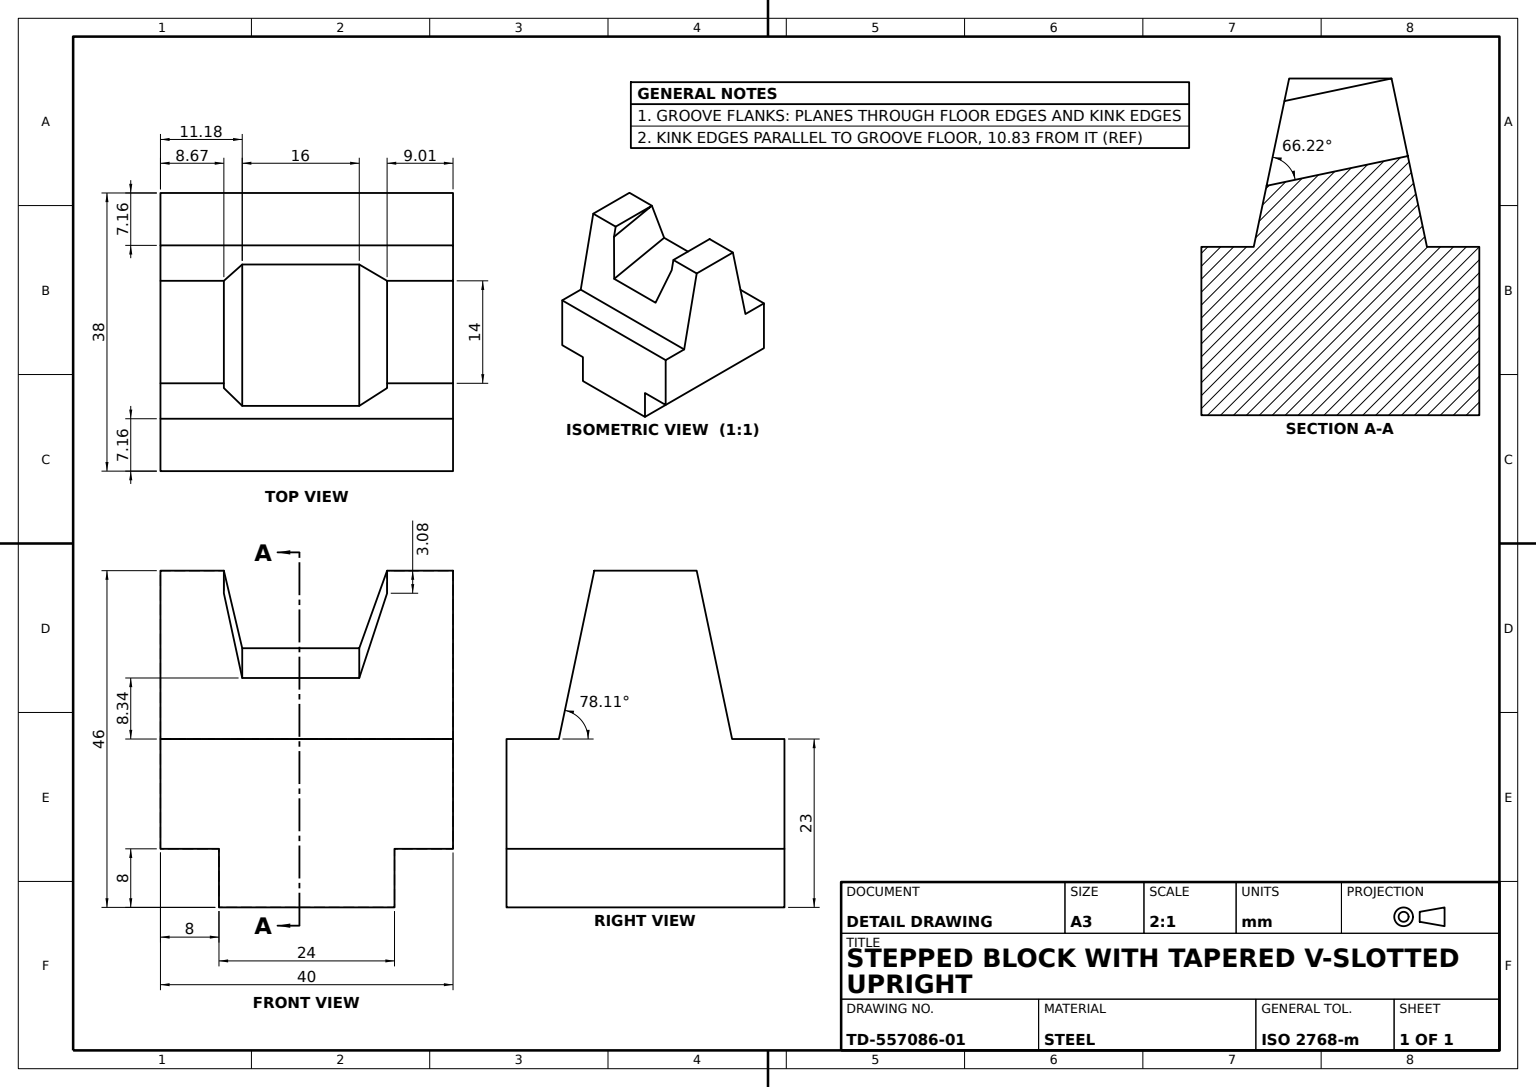
SolidWorks part; units mm, degrees
material "Plain Carbon Steel"
ref_plane "Front Plane" through (0, 0, 0) normal (0, 0, 1) x (1, 0, 0)
ref_plane "Top Plane" through (0, 0, 0) normal (0, 1, 0) x (1, 0, 0)
ref_plane "Right Plane" through (0, 0, 0) normal (1, 0, 0) x (0, 0, -1)
sketch "Base Profile Sketch" plane through (0, 0, 0) normal (0, 0, 1) x (1, 0, 0)
  line L1 (-20, 23) -> (20, 23)
  line L2 (-20, 23) -> (-20, -23)
  line L3 (-20, -23) -> (20, -23)
  line L4 (20, 23) -> (20, -23)
  line L5 (-20, 23) -> (20, -23) construction
  line L6 (-20, -23) -> (20, 23) construction
  point P0 (0, 0)
  dimension "D1" = 40
  dimension "D2" = 46
extrude "Base Block" add sketch "Base Profile Sketch" along normal blind 38
sketch "Bottom Step Sketch" plane through (0, 0, 38) normal (0, 0, 1) x (1, 0, 0)
  line L0 (-12, -23) -> (12, -23)
  line L2 (12, -23) -> (20, -23)
  line L3 (-20, -23) -> (-20, -15)
  line L4 (-12, -23) -> (11.2141, -23)
  line L5 (-12, -23) -> (-12, 0)
  line L6 (-12, 0) -> (11.2141, 0)
  line L7 (11.2141, -23) -> (11.2141, 0)
  line L9 (-20, -15) -> (-12, -15)
  line L10 (-12, -15) -> (-12, -23)
  line L12 (20, 23) -> (-20, 23) construction
  line M3 (-20, 23) -> (-20, -23)
  line M4 (-20, -23) -> (20, -23)
  dimension "D1" = 8
  dimension "D2" = 24
  dimension "D3" = 23
  dimension "D4" = 8
  dimension "D5" = 40
  dimension "D6" = 8
  dimension "D7" = 0.7859
  dimension "D8" = 46
extrude "Bottom Step Cut" cut sketch "Bottom Step Sketch" against normal through all contours L9 L5 M3 M4
sketch "Corner Notch Sketch" plane through (0, 0, 38) normal (0, 0, 1) x (1, 0, 0)
  line L0 (20, -23) -> (12, -23)
  line L1 (-12, -23) -> (20, -23) construction
  line L2 (12, -23) -> (12, -15)
  line L3 (12, -15) -> (20, -15)
  line L4 (20, -23) -> (20, 23) construction
  line L5 (20, -23) -> (20, -15)
  dimension "D1" = 8
  dimension "D2" = 8
extrude "Corner Notch 8x8" cut sketch "Corner Notch Sketch" against normal through all
sketch "V-Groove Reference Sketch" plane through (0, 0, 0) normal (1, 0, 0) x (0, 0, -1)
  line L0 (-19, 23) -> (-26, 23)
  line L1 (-38, 23) -> (0, 23) construction
  line L2 (-19, 23) -> (-12, 23)
  dimension "D1" = 7
  dimension "D2" = 7
sketch "V-Groove Profile Sketch" plane through (0, 0, 0) normal (1, 0, 0) x (0, 0, -1)
  line L0 (-19, -15) -> (-34, -15)
  line L1 (0, -15) -> (-38, -15) construction
  line L2 (-34, -15) -> (-4, -15)
  line L3 (-26, 23) -> (-34, -15)
  line L4 (-4, -15) -> (-12, 23)
  line L5 (-38, -23) -> (-38, 0)
  line L6 (-38, -15) -> (-38, 23) construction
  line L7 (-38, 0) -> (-30.8421, 0)
  line L8 (-7.1579, 0) -> (0, 0)
  line L9 (0, 0) -> (0, -23)
  line L10 (-38, 0) -> (-38, 23)
  line L11 (-38, 23) -> (-26, 23)
  line L12 (-12, 23) -> (0, 23)
  line L13 (0, 23) -> (0, 0)
  dimension "D1" = 15
  dimension "D2" = 15
extrude "V-Groove Cut" cut sketch "V-Groove Profile Sketch" against normal mid plane 92 contours L11 L10 L7 L3 | L13 L12 L4 L8
sketch "Slot Sketch" plane through (0, -1.443, 6.8541) normal (0, 0.206, -0.9785) x (-1, 0, 0)
  line L0 (-12, 27.8629) -> (-20, 27.8629)
  line L1 (-20, 27.8629) -> (20, 27.8629) construction
  line L2 (20, 27.8629) -> (12, 27.8629)
  line L3 (0.82, 14.1511) -> (8.82, 14.1511)
  line L4 (8.82, 14.1511) -> (-7.18, 14.1511)
  line L5 (-7.18, 14.1511) -> (-12, 27.8629)
  line L6 (8.82, 14.1511) -> (12, 27.8629)
  line L7 (-12, 27.8629) -> (12, 27.8629)
  line L8 (-12, 27.8629) -> (12, 27.8629)
  line L9 (20, 1.4746) -> (20, 24.9788) construction
  line L10 (20, 24.9788) -> (-20, 24.9788) construction
  line M2 (20, 24.9788) -> (-20, 24.9788)
  dimension "D1" = 8
  dimension "D2" = 8
  dimension "D3" = 11.18
  dimension "D4" = 10.8277
extrude "Slot Cut 8x8" cut sketch "Slot Sketch" against normal mid plane 92 contours L3 L6 L5 L4 M2
sketch "Side Trim Sketch" plane through (0, -1.443, 6.8541) normal (0, 0.206, -0.9785) x (-1, 0, 0)
  line L0 (-20, 24.9788) -> (-20, 1.4746) construction
  line L1 (-10.9862, 24.9788) -> (11.3311, 24.9788)
  line L2 (-10.9862, 24.9788) -> (-10.9862, 29.6486)
  line L3 (-10.9862, 29.6486) -> (11.3311, 29.6486)
  line L4 (11.3311, 24.9788) -> (11.3311, 29.6486)
  line L5 (-10.9862, 24.9788) -> (-20, 24.9788) construction
  dimension "D1" = 31.3311
  dimension "D2" = 4.6698
extrude "Side Trim Cut" cut sketch "Side Trim Sketch" against normal mid plane 92
